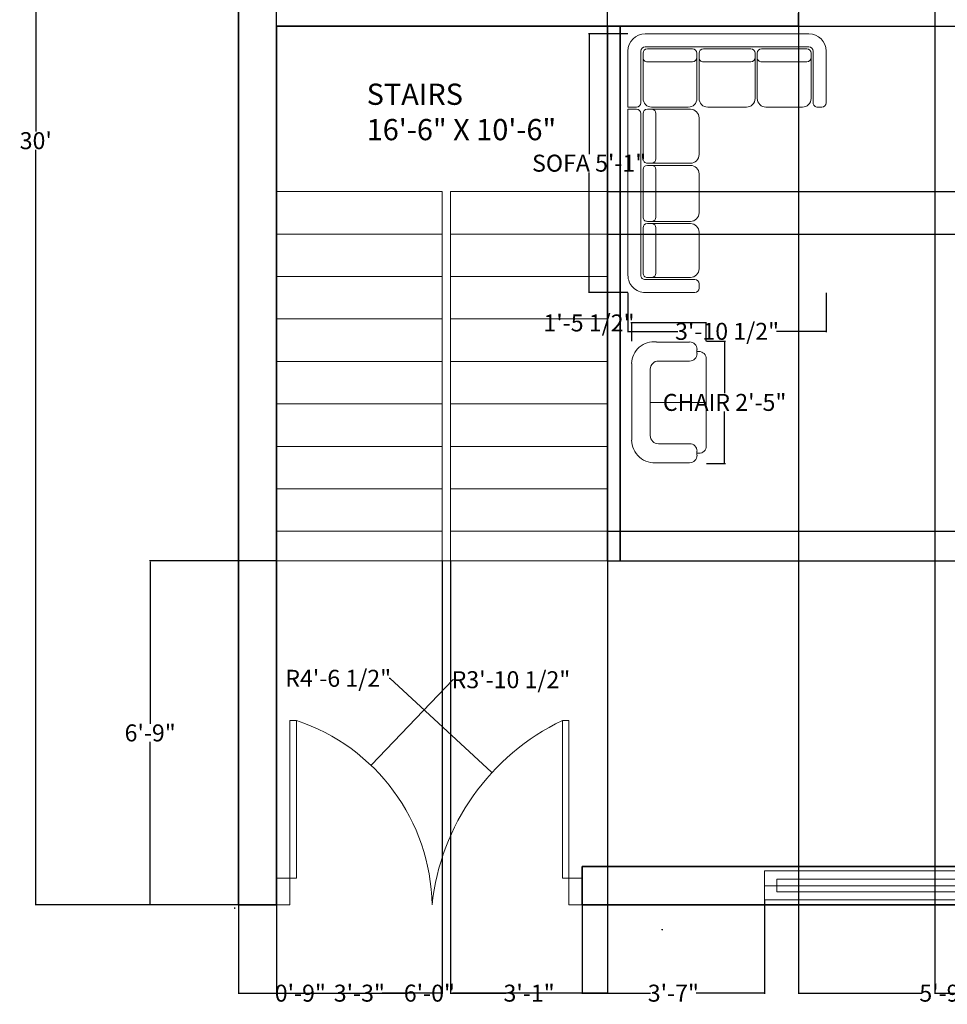
# Model space of a CAD drawing. Units: inches. Extents: x 311 to 754, y 60 to 497.
# Tile 1 of 11: x 311 to 530, y 64 to 296. Entities that reach past the tile are written whole.
import ezdxf

# ---------------------------------------------------------------- set-up
doc = ezdxf.new("R2010")
doc.units = ezdxf.units.IN
doc.header["$MEASUREMENT"] = 0
for name, color, linetype, lineweight in [('A-ANNO-DIMS', 2, 'Continuous', 18), ('A-AREA-IDEN', 1, 'Continuous', 18), ('A-FURN', 70, 'Continuous', 13), ('A-WALL', 7, 'Continuous', 35), ('doors', 210, 'Continuous', 18), ('stairs', 130, 'Continuous', 18), ('windows', 120, 'Continuous', 18)]:
    doc.layers.add(name, color=color, linetype=linetype, lineweight=lineweight)
doc.styles.get("Standard").update_dxf_attribs({"font": 'arial.ttf'})
doc.dimstyles.get("Standard").update_dxf_attribs({"dimtxt": 4, "dimasz": 0.18, "dimexe": 0.18, "dimexo": 0.0625, "dimgap": 0.09, "dimtad": 0, "dimtih": 1, "dimtoh": 1, "dimdec": 0, "dimrnd": 6, "dimzin": 0, "dimdsep": 46, "dimlunit": 3, "dimtxsty": 'Standard', "dimcen": 0.09, "dimadec": 0, "dimazin": 0, "dimtfac": 1, "dimtdec": 0, "dimtofl": 0, "dimtmove": 0, "dimatfit": 3, "dimfxl": 1, "dimtolj": 1, "dimtzin": 0, "dimarcsym": 0})

# ---------------------------------------------------------------- blocks, each defined once
blk = doc.blocks.new('A$C2AFA021D')
for p, q in [((0.8, 2.3), (0.2, 2.3)), ((0.85, 2.2), (0.85, 2.25)), ((0, 2.1), (0, 0.2)), ((0.15, 0.2), (0.15, 2.1)), ((0.175, 1.55), (0.175, 2.075)), ((0.2, 2.15), (0.8, 2.15)), ((0.225, 2.125), (0.275, 2.125)), ((0.75, 2.125), (0.275, 2.125)), ((0.325, 2.075), (0.325, 1.55)), ((0.85, 1.6), (0.85, 2.025)), ((0.275, 1.5), (0.225, 1.5)), ((0.275, 1.5), (0.75, 1.5)), ((0.175, 0.875), (0.175, 1.425)), ((0.225, 1.475), (0.275, 1.475)), ((0.75, 1.475), (0.275, 1.475)), ((0.325, 1.425), (0.325, 0.875)), ((0.85, 0.925), (0.85, 1.375)), ((0.275, 0.825), (0.225, 0.825)), ((0.225, 0.8), (0.275, 0.8)), ((0.275, 0.825), (0.75, 0.825)), ((0.75, 0.8), (0.275, 0.8)), ((0.975, 0.825), (1.4, 0.825)), ((1.625, 0.825), (2.075, 0.825)), ((2.3, 0.825), (2.725, 0.825)), ((2.9, 0.825), (2.95, 0.825)), ((0.175, 0.225), (0.175, 0.75)), ((0.325, 0.75), (0.325, 0.225)), ((0.85, 0.275), (0.85, 0.7)), ((0.875, 0.275), (0.875, 0.725)), ((1.5, 0.725), (1.5, 0.275)), ((1.525, 0.275), (1.525, 0.725)), ((2.175, 0.725), (2.175, 0.275)), ((2.2, 0.275), (2.2, 0.725)), ((2.825, 0.725), (2.825, 0.275)), ((2.85, 0.2), (2.85, 0.775)), ((3, 0.775), (3, 0.2)), ((0.875, 0.275), (0.875, 0.225)), ((1.45, 0.325), (0.925, 0.325)), ((1.5, 0.225), (1.5, 0.275)), ((1.525, 0.275), (1.525, 0.225)), ((2.125, 0.325), (1.575, 0.325)), ((2.175, 0.225), (2.175, 0.275)), ((2.2, 0.275), (2.2, 0.225)), ((2.775, 0.325), (2.25, 0.325)), ((2.825, 0.225), (2.825, 0.275)), ((0.8, 0.15), (0.2, 0.15)), ((0.275, 0.175), (0.225, 0.175)), ((0.275, 0.175), (0.75, 0.175)), ((0.925, 0.175), (1.45, 0.175)), ((0.925, 0.15), (2.8, 0.15)), ((1.575, 0.175), (2.125, 0.175)), ((2.25, 0.175), (2.775, 0.175)), ((0.85, 0), (0.85, 0.1)), ((0.875, 0.1), (0.875, 0)), ((0.2, 0), (0.85, 0)), ((2.8, 0), (0.875, 0))]:
    blk.add_line(p, q)
for centre, radius, start, end in [((0.2, 2.1), 0.2, 90, 180), ((0.8, 2.25), 0.05, 0, 90), ((0.8, 2.2), 0.05, 270, 0), ((0.2, 2.1), 0.05, 90, 180), ((0.225, 2.075), 0.05, 90, 180), ((0.275, 2.075), 0.05, 0, 90), ((0.75, 2.025), 0.1, 0, 90), ((0.75, 1.6), 0.1, 270, 0), ((0.225, 1.55), 0.05, 180, 270), ((0.275, 1.55), 0.05, 270, 0), ((0.225, 1.425), 0.05, 90, 180), ((0.275, 1.425), 0.05, 0, 90), ((0.75, 1.375), 0.1, 360, 90), ((0.75, 0.925), 0.1, 270, 0), ((0.225, 0.875), 0.05, 180, 270), ((0.225, 0.75), 0.05, 90, 180), ((0.275, 0.875), 0.05, 270, 0), ((0.275, 0.75), 0.05, 0, 90), ((0.75, 0.7), 0.1, 0, 90), ((0.975, 0.725), 0.1, 90, 180), ((1.4, 0.725), 0.1, 0, 90), ((1.625, 0.725), 0.1, 90, 180), ((2.075, 0.725), 0.1, 0, 90), ((2.3, 0.725), 0.1, 90, 180), ((2.725, 0.725), 0.1, 0, 90), ((2.9, 0.775), 0.05, 90, 180), ((2.95, 0.775), 0.05, 0, 90), ((0.75, 0.275), 0.1, 270, 0), ((0.925, 0.275), 0.05, 90, 180), ((1.45, 0.275), 0.05, 360, 90), ((1.575, 0.275), 0.05, 90, 180), ((2.125, 0.275), 0.05, 360, 90), ((2.25, 0.275), 0.05, 90, 180), ((2.775, 0.275), 0.05, 360, 90), ((0.2, 0.2), 0.2, 180, 270), ((0.2, 0.2), 0.05, 180, 270), ((0.225, 0.225), 0.05, 180, 270), ((0.275, 0.225), 0.05, 270, 0), ((0.8, 0.1), 0.05, 0, 90), ((0.925, 0.225), 0.05, 180, 270), ((0.925, 0.1), 0.05, 90, 180), ((1.45, 0.225), 0.05, 270, 0), ((1.575, 0.225), 0.05, 180, 270), ((2.125, 0.225), 0.05, 270, 0), ((2.25, 0.225), 0.05, 180, 270), ((2.775, 0.225), 0.05, 270, 0), ((2.8, 0.2), 0.2, 270, 0), ((2.8, 0.2), 0.05, 270, 0)]:
    blk.add_arc(centre, radius, start, end)
blk = doc.blocks.new('A$C6D011943')
for p, q in [((1.448, 1.089), (0.332, 1.089)), ((1.364, 0.818), (0.398, 0.818)), ((0.881, 0.818), (0.881, 0)), ((1.762, 0.247), (1.762, 0.727)), ((0, 0.709), (0, 0.247)), ((0.278, 0.697), (0.278, 0.244)), ((1.485, 0.244), (1.485, 0.697)), ((0.109, 0.136), (0.169, 0.136)), ((0.139, 0.109), (0.139, 0.136)), ((1.515, 0), (0.247, 0)), ((1.593, 0.136), (1.654, 0.136)), ((1.648, 0.136), (1.623, 0.136)), ((1.623, 0.109), (1.623, 0.136))]:
    blk.add_line(p, q)
for centre, radius, start, end in [((0.339, 0.748), 0.342, 91.2564, 186.501), ((1.441, 0.766), 0.324, 353.159, 88.6697), ((0.398, 0.697), 0.121, 90, 180), ((1.364, 0.697), 0.121, 0, 90), ((0.109, 0.244), 0.109, 180, 270), ((0.169, 0.244), 0.109, 270, 0), ((1.593, 0.244), 0.109, 180, 270), ((1.654, 0.244), 0.109, 270, 0), ((0.247, 0.109), 0.109, 180, 270), ((1.515, 0.109), 0.109, 270, 0)]:
    blk.add_arc(centre, radius, start, end)
blk = doc.blocks.new('*D104')
at = {"layer": 'A-ANNO-DIMS', "color": 0, "lineweight": -2, "transparency": 16777216}
for p, q in [((362.74, 447.24), (314.86, 447.24)), ((315.04, 447.06), (315.04, 269.37)), ((315.04, 87.42), (315.04, 265.1)), ((362.74, 87.24), (314.86, 87.24))]:
    blk.add_line(p, q, dxfattribs=at)
at = {"layer": 'A-ANNO-DIMS', "color": 0, "transparency": 16777216}
for points in [[(315.01, 447.06), (315.07, 447.06), (315.04, 447.24)], [(315.01, 87.42), (315.07, 87.42), (315.04, 87.24)]]:
    blk.add_solid(points, dxfattribs=at)
at = {"layer": 'Defpoints', "color": 0, "transparency": 16777216}
for p in [(362.8, 447.24), (315.04, 87.24), (362.8, 87.24)]:
    blk.add_point(p, dxfattribs=at)
at = {"layer": 'A-ANNO-DIMS', "color": 0, "transparency": 16777216, "insert": (315.04, 267.24), "char_height": 4, "attachment_point": 5}
blk.add_mtext("\\A1;30'", dxfattribs=at)
blk = doc.blocks.new('WIN-FRAME-59IN')
for points in [[(0, 0), (0, 6.8), (58.92, 6.8), (58.92, 0)], [(2.85, 4.84), (55.97, 4.84), (55.97, 1.89), (2.85, 1.89)]]:
    blk.add_lwpolyline(points, close=True)
blk = doc.blocks.new('*D114')
at = {"layer": 'A-ANNO-DIMS', "color": 0, "lineweight": -2, "transparency": 16777216}
for p, q in [((454.54, 292.4), (445.28, 292.4)), ((445.46, 292.22), (445.46, 264.1)), ((445.46, 231.65), (445.46, 259.78)), ((454.54, 231.47), (445.28, 231.47))]:
    blk.add_line(p, q, dxfattribs=at)
at = {"layer": 'A-ANNO-DIMS', "color": 0, "transparency": 16777216}
for points in [[(445.43, 292.22), (445.49, 292.22), (445.46, 292.4)], [(445.43, 231.65), (445.49, 231.65), (445.46, 231.47)]]:
    blk.add_solid(points, dxfattribs=at)
at = {"layer": 'Defpoints', "color": 0, "transparency": 16777216}
for p in [(454.6, 292.4), (445.46, 231.47), (454.6, 231.47)]:
    blk.add_point(p, dxfattribs=at)
at = {"layer": 'A-ANNO-DIMS', "color": 0, "transparency": 16777216, "insert": (445.46, 261.94), "char_height": 4, "attachment_point": 5}
blk.add_mtext('\\A1;SOFA 5\'-1"', dxfattribs=at)
blk = doc.blocks.new('*D115')
at = {"layer": 'A-ANNO-DIMS', "color": 0, "lineweight": -2, "transparency": 16777216}
for p, q in [((454.6, 231.41), (454.6, 222.15)), ((501.31, 231.41), (501.31, 222.15)), ((454.78, 222.33), (466.34, 222.33)), ((501.13, 222.33), (489.58, 222.33))]:
    blk.add_line(p, q, dxfattribs=at)
at = {"layer": 'A-ANNO-DIMS', "color": 0, "transparency": 16777216}
for points in [[(454.78, 222.36), (454.78, 222.3), (454.6, 222.33)], [(501.13, 222.36), (501.13, 222.3), (501.31, 222.33)]]:
    blk.add_solid(points, dxfattribs=at)
at = {"layer": 'Defpoints', "color": 0, "transparency": 16777216}
for p in [(454.6, 231.47), (501.31, 231.47), (501.31, 222.33)]:
    blk.add_point(p, dxfattribs=at)
at = {"layer": 'A-ANNO-DIMS', "color": 0, "transparency": 16777216, "insert": (477.96, 222.33), "char_height": 4, "attachment_point": 5}
blk.add_mtext('\\A1;3\'-10 1/2"', dxfattribs=at)
blk = doc.blocks.new('*D116')
at = {"layer": 'A-ANNO-DIMS', "color": 0, "lineweight": -2, "transparency": 16777216}
for p, q in [((473.13, 219.99), (477.56, 219.99)), ((477.38, 219.81), (477.38, 207.75)), ((477.38, 191.37), (477.38, 203.43)), ((473.13, 191.19), (477.56, 191.19))]:
    blk.add_line(p, q, dxfattribs=at)
at = {"layer": 'A-ANNO-DIMS', "color": 0, "transparency": 16777216}
for points in [[(477.35, 219.81), (477.41, 219.81), (477.38, 219.99)], [(477.35, 191.37), (477.41, 191.37), (477.38, 191.19)]]:
    blk.add_solid(points, dxfattribs=at)
at = {"layer": 'Defpoints', "color": 0, "transparency": 16777216}
for p in [(473.06, 219.99), (477.38, 219.99), (473.06, 191.19)]:
    blk.add_point(p, dxfattribs=at)
at = {"layer": 'A-ANNO-DIMS', "color": 0, "transparency": 16777216, "insert": (477.38, 205.59), "char_height": 4, "attachment_point": 5}
blk.add_mtext('\\A1;CHAIR 2\'-5"', dxfattribs=at)
blk = doc.blocks.new('*D117')
at = {"layer": 'A-ANNO-DIMS', "color": 0, "lineweight": -2, "transparency": 16777216}
for p, q in [((455.48, 224.31), (455.3, 224.31)), ((455.48, 220.05), (455.48, 224.49)), ((472.88, 224.31), (455.66, 224.31)), ((473.06, 220.05), (473.06, 224.49))]:
    blk.add_line(p, q, dxfattribs=at)
at = {"layer": 'A-ANNO-DIMS', "color": 0, "transparency": 16777216}
for points in [[(455.66, 224.34), (455.66, 224.28), (455.48, 224.31)], [(472.88, 224.34), (472.88, 224.28), (473.06, 224.31)]]:
    blk.add_solid(points, dxfattribs=at)
at = {"layer": 'Defpoints', "color": 0, "transparency": 16777216}
for p in [(455.48, 224.31), (455.48, 219.99), (473.06, 219.99)]:
    blk.add_point(p, dxfattribs=at)
at = {"layer": 'A-ANNO-DIMS', "color": 0, "transparency": 16777216, "insert": (445.42, 224.31), "char_height": 4, "attachment_point": 5}
blk.add_mtext('\\A1;1\'-5 1/2"', dxfattribs=at)
blk = doc.blocks.new('*D125')
at = {"layer": 'A-ANNO-DIMS', "color": 0, "lineweight": -2, "transparency": 16777216}
for p, q in [((371.8, 87.18), (371.8, 66.26)), ((443.8, 87.18), (443.8, 66.26)), ((371.98, 66.44), (402.39, 66.44)), ((443.62, 66.44), (413.22, 66.44))]:
    blk.add_line(p, q, dxfattribs=at)
at = {"layer": 'A-ANNO-DIMS', "color": 0, "transparency": 16777216}
for points in [[(371.98, 66.47), (371.98, 66.41), (371.8, 66.44)], [(443.62, 66.47), (443.62, 66.41), (443.8, 66.44)]]:
    blk.add_solid(points, dxfattribs=at)
at = {"layer": 'Defpoints', "color": 0, "transparency": 16777216}
for p in [(371.8, 87.24), (443.8, 87.24), (443.8, 66.44)]:
    blk.add_point(p, dxfattribs=at)
at = {"layer": 'A-ANNO-DIMS', "color": 0, "transparency": 16777216, "insert": (407.8, 66.44), "char_height": 4, "attachment_point": 5}
blk.add_mtext('\\A1;6\'-0"', dxfattribs=at)
blk = doc.blocks.new('*D126')
at = {"layer": 'A-ANNO-DIMS', "color": 0, "lineweight": -2, "transparency": 16777216}
for p, q in [((486.8, 88.36), (486.8, 66.26)), ((443.8, 87.18), (443.8, 66.26)), ((443.98, 66.44), (459.9, 66.44)), ((486.62, 66.44), (470.71, 66.44))]:
    blk.add_line(p, q, dxfattribs=at)
at = {"layer": 'A-ANNO-DIMS', "color": 0, "transparency": 16777216}
for points in [[(443.98, 66.47), (443.98, 66.41), (443.8, 66.44)], [(486.62, 66.47), (486.62, 66.41), (486.8, 66.44)]]:
    blk.add_solid(points, dxfattribs=at)
at = {"layer": 'Defpoints', "color": 0, "transparency": 16777216}
for p in [(486.8, 88.42), (443.8, 87.24), (486.8, 66.44)]:
    blk.add_point(p, dxfattribs=at)
at = {"layer": 'A-ANNO-DIMS', "color": 0, "transparency": 16777216, "insert": (465.3, 66.44), "char_height": 4, "attachment_point": 5}
blk.add_mtext('\\A1;3\'-7"', dxfattribs=at)
blk = doc.blocks.new('*D127')
at = {"layer": 'A-ANNO-DIMS', "color": 0, "lineweight": -2, "transparency": 16777216}
for p, q in [((371.74, 168.24), (341.82, 168.24)), ((342, 168.06), (342, 129.87)), ((342, 87.42), (342, 125.61)), ((362.74, 87.24), (341.82, 87.24))]:
    blk.add_line(p, q, dxfattribs=at)
at = {"layer": 'A-ANNO-DIMS', "color": 0, "transparency": 16777216}
for points in [[(341.97, 168.06), (342.03, 168.06), (342, 168.24)], [(341.97, 87.42), (342.03, 87.42), (342, 87.24)]]:
    blk.add_solid(points, dxfattribs=at)
at = {"layer": 'Defpoints', "color": 0, "transparency": 16777216}
for p in [(342, 168.24), (371.8, 168.24), (362.8, 87.24)]:
    blk.add_point(p, dxfattribs=at)
at = {"layer": 'A-ANNO-DIMS', "color": 0, "transparency": 16777216, "insert": (342, 127.74), "char_height": 4, "attachment_point": 5}
blk.add_mtext('\\A1;6\'-9"', dxfattribs=at)
blk = doc.blocks.new('*D128')
at = {"layer": 'A-ANNO-DIMS', "color": 0, "lineweight": -2, "transparency": 16777216}
for p, q in [((362.8, 87.18), (362.8, 66.26)), ((371.8, 87.18), (371.8, 66.26)), ((362.98, 66.44), (371.62, 66.44)), ((371.8, 66.44), (371.98, 66.44))]:
    blk.add_line(p, q, dxfattribs=at)
at = {"layer": 'A-ANNO-DIMS', "color": 0, "transparency": 16777216}
for points in [[(362.98, 66.47), (362.98, 66.41), (362.8, 66.44)], [(371.62, 66.47), (371.62, 66.41), (371.8, 66.44)]]:
    blk.add_solid(points, dxfattribs=at)
at = {"layer": 'Defpoints', "color": 0, "transparency": 16777216}
for p in [(362.8, 87.24), (371.8, 87.24), (371.8, 66.44)]:
    blk.add_point(p, dxfattribs=at)
at = {"layer": 'A-ANNO-DIMS', "color": 0, "transparency": 16777216, "insert": (377.39, 66.44), "char_height": 4, "attachment_point": 5}
blk.add_mtext('\\A1;0\'-9"', dxfattribs=at)
blk = doc.blocks.new('*D132')
at = {"layer": 'A-ANNO-DIMS', "color": 0, "lineweight": -2, "transparency": 16777216}
for p, q in [((526.91, 339.18), (526.91, 66.26)), ((560.82, 339.18), (560.82, 66.26)), ((527.09, 66.44), (536.87, 66.44)), ((560.64, 66.44), (550.86, 66.44))]:
    blk.add_line(p, q, dxfattribs=at)
at = {"layer": 'A-ANNO-DIMS', "color": 0, "transparency": 16777216}
for points in [[(527.09, 66.47), (527.09, 66.41), (526.91, 66.44)], [(560.64, 66.47), (560.64, 66.41), (560.82, 66.44)]]:
    blk.add_solid(points, dxfattribs=at)
at = {"layer": 'Defpoints', "color": 0, "transparency": 16777216}
for p in [(526.91, 339.24), (560.82, 339.24), (526.91, 66.44)]:
    blk.add_point(p, dxfattribs=at)
at = {"layer": 'A-ANNO-DIMS', "color": 0, "transparency": 16777216, "insert": (543.87, 66.44), "char_height": 4, "attachment_point": 5}
blk.add_mtext('\\A1;2\'-10"', dxfattribs=at)
blk = doc.blocks.new('*D134')
at = {"layer": 'A-ANNO-DIMS', "color": 0, "lineweight": -2, "transparency": 16777216}
for p, q in [((494.8, 342.18), (494.8, 66.26)), ((563.8, 342.18), (563.8, 66.26)), ((494.98, 66.44), (523.9, 66.44)), ((563.62, 66.44), (534.71, 66.44))]:
    blk.add_line(p, q, dxfattribs=at)
at = {"layer": 'A-ANNO-DIMS', "color": 0, "transparency": 16777216}
for points in [[(494.98, 66.47), (494.98, 66.41), (494.8, 66.44)], [(563.62, 66.47), (563.62, 66.41), (563.8, 66.44)]]:
    blk.add_solid(points, dxfattribs=at)
at = {"layer": 'Defpoints', "color": 0, "transparency": 16777216}
for p in [(494.8, 342.24), (563.8, 342.24), (563.8, 66.44)]:
    blk.add_point(p, dxfattribs=at)
at = {"layer": 'A-ANNO-DIMS', "color": 0, "transparency": 16777216, "insert": (529.3, 66.44), "char_height": 4, "attachment_point": 5}
blk.add_mtext('\\A1;5\'-9"', dxfattribs=at)
blk = doc.blocks.new('*D136')
at = {"layer": 'A-ANNO-DIMS', "color": 0, "lineweight": -2, "transparency": 16777216}
for p, q in [((371.8, 294.3), (371.8, 486.86)), ((371.98, 486.68), (405.39, 486.68)), ((449.62, 486.68), (416.22, 486.68)), ((449.8, 294.3), (449.8, 486.86))]:
    blk.add_line(p, q, dxfattribs=at)
at = {"layer": 'A-ANNO-DIMS', "color": 0, "transparency": 16777216}
for points in [[(371.98, 486.71), (371.98, 486.65), (371.8, 486.68)], [(449.62, 486.71), (449.62, 486.65), (449.8, 486.68)]]:
    blk.add_solid(points, dxfattribs=at)
at = {"layer": 'Defpoints', "color": 0, "transparency": 16777216}
for p in [(371.8, 486.68), (371.8, 294.24), (449.8, 294.24)]:
    blk.add_point(p, dxfattribs=at)
at = {"layer": 'A-ANNO-DIMS', "color": 0, "transparency": 16777216, "insert": (410.8, 486.68), "char_height": 4, "attachment_point": 5}
blk.add_mtext('\\A1;6\'-6"', dxfattribs=at)
blk = doc.blocks.new('*D137')
at = {"layer": 'A-ANNO-DIMS', "color": 0, "lineweight": -2, "transparency": 16777216}
for p, q in [((371.8, 168.18), (371.8, 66.26)), ((410.8, 168.18), (410.8, 66.26)), ((371.98, 66.44), (385.9, 66.44)), ((410.62, 66.44), (396.71, 66.44))]:
    blk.add_line(p, q, dxfattribs=at)
at = {"layer": 'A-ANNO-DIMS', "color": 0, "transparency": 16777216}
for points in [[(371.98, 66.47), (371.98, 66.41), (371.8, 66.44)], [(410.62, 66.47), (410.62, 66.41), (410.8, 66.44)]]:
    blk.add_solid(points, dxfattribs=at)
at = {"layer": 'Defpoints', "color": 0, "transparency": 16777216}
for p in [(371.8, 168.24), (410.8, 168.24), (371.8, 66.44)]:
    blk.add_point(p, dxfattribs=at)
at = {"layer": 'A-ANNO-DIMS', "color": 0, "transparency": 16777216, "insert": (391.3, 66.44), "char_height": 4, "attachment_point": 5}
blk.add_mtext('\\A1;3\'-3"', dxfattribs=at)
blk = doc.blocks.new('*D138')
at = {"layer": 'A-ANNO-DIMS', "color": 0, "lineweight": -2, "transparency": 16777216}
for p, q in [((412.8, 168.18), (412.8, 66.26)), ((449.8, 168.18), (449.8, 66.26)), ((412.98, 66.44), (425.9, 66.44)), ((449.62, 66.44), (436.71, 66.44))]:
    blk.add_line(p, q, dxfattribs=at)
at = {"layer": 'A-ANNO-DIMS', "color": 0, "transparency": 16777216}
for points in [[(412.98, 66.47), (412.98, 66.41), (412.8, 66.44)], [(449.62, 66.47), (449.62, 66.41), (449.8, 66.44)]]:
    blk.add_solid(points, dxfattribs=at)
at = {"layer": 'Defpoints', "color": 0, "transparency": 16777216}
for p in [(412.8, 168.24), (449.8, 168.24), (449.8, 66.44)]:
    blk.add_point(p, dxfattribs=at)
at = {"layer": 'A-ANNO-DIMS', "color": 0, "transparency": 16777216, "insert": (431.3, 66.44), "char_height": 4, "attachment_point": 5}
blk.add_mtext('\\A1;3\'-1"', dxfattribs=at)
blk = doc.blocks.new('*D139')
at = {"layer": 'A-ANNO-DIMS', "color": 0, "lineweight": -2, "transparency": 16777216}
for p, q in [((449.87, 255.24), (743.78, 255.24)), ((743.6, 255.06), (743.6, 252.37)), ((743.6, 245.42), (743.6, 248.11)), ((449.87, 245.24), (743.78, 245.24))]:
    blk.add_line(p, q, dxfattribs=at)
at = {"layer": 'A-ANNO-DIMS', "color": 0, "transparency": 16777216}
for points in [[(743.57, 255.06), (743.63, 255.06), (743.6, 255.24)], [(743.57, 245.42), (743.63, 245.42), (743.6, 245.24)]]:
    blk.add_solid(points, dxfattribs=at)
at = {"layer": 'Defpoints', "color": 0, "transparency": 16777216}
for p in [(449.8, 255.24), (743.6, 255.24), (449.8, 245.24)]:
    blk.add_point(p, dxfattribs=at)
at = {"layer": 'A-ANNO-DIMS', "color": 0, "transparency": 16777216, "insert": (743.6, 250.24), "char_height": 4, "attachment_point": 5}
blk.add_mtext('\\A1;0\'-10"', dxfattribs=at)
blk = doc.blocks.new('*D140')
at = {"layer": 'A-ANNO-DIMS', "color": 0, "lineweight": -2, "transparency": 16777216}
for p, q in [((449.87, 294.24), (743.78, 294.24)), ((743.6, 294.06), (743.6, 276.87)), ((743.6, 255.42), (743.6, 272.6)), ((449.87, 255.24), (743.78, 255.24))]:
    blk.add_line(p, q, dxfattribs=at)
at = {"layer": 'A-ANNO-DIMS', "color": 0, "transparency": 16777216}
for points in [[(743.57, 294.06), (743.63, 294.06), (743.6, 294.24)], [(743.57, 255.42), (743.63, 255.42), (743.6, 255.24)]]:
    blk.add_solid(points, dxfattribs=at)
at = {"layer": 'Defpoints', "color": 0, "transparency": 16777216}
for p in [(449.8, 294.24), (743.6, 294.24), (449.8, 255.24)]:
    blk.add_point(p, dxfattribs=at)
at = {"layer": 'A-ANNO-DIMS', "color": 0, "transparency": 16777216, "insert": (743.6, 274.74), "char_height": 4, "attachment_point": 5}
blk.add_mtext('\\A1;3\'-3"', dxfattribs=at)
blk = doc.blocks.new('*D141')
at = {"layer": 'A-ANNO-DIMS', "color": 0, "lineweight": -2, "transparency": 16777216}
for p, q in [((449.87, 175.24), (743.78, 175.24)), ((743.6, 175.06), (743.6, 173.87)), ((743.6, 168.42), (743.6, 169.61)), ((449.87, 168.24), (743.78, 168.24))]:
    blk.add_line(p, q, dxfattribs=at)
at = {"layer": 'A-ANNO-DIMS', "color": 0, "transparency": 16777216}
for points in [[(743.57, 175.06), (743.63, 175.06), (743.6, 175.24)], [(743.57, 168.42), (743.63, 168.42), (743.6, 168.24)]]:
    blk.add_solid(points, dxfattribs=at)
at = {"layer": 'Defpoints', "color": 0, "transparency": 16777216}
for p in [(449.8, 175.24), (743.6, 175.24), (449.8, 168.24)]:
    blk.add_point(p, dxfattribs=at)
at = {"layer": 'A-ANNO-DIMS', "color": 0, "transparency": 16777216, "insert": (743.6, 171.74), "char_height": 4, "attachment_point": 5}
blk.add_mtext('\\A1;0\'-7"', dxfattribs=at)
blk = doc.blocks.new('*D157')
at = {"layer": 'A-ANNO-DIMS', "color": 0, "lineweight": -2, "transparency": 16777216}
for p, q in [((413.32, 140.27), (394.18, 120.23)), ((413.5, 140.27), (413.32, 140.27)), ((361.86, 86.49), (362.04, 86.49)), ((361.95, 86.4), (361.95, 86.58))]:
    blk.add_line(p, q, dxfattribs=at)
at = {"layer": 'A-ANNO-DIMS', "color": 0, "transparency": 16777216}
blk.add_solid([(394.16, 120.26), (394.2, 120.21), (394.05, 120.1)], dxfattribs=at)
at = {"layer": 'Defpoints', "color": 0, "transparency": 16777216}
for p in [(394.05, 120.1), (361.95, 86.49)]:
    blk.add_point(p, dxfattribs=at)
at = {"layer": 'A-ANNO-DIMS', "color": 0, "transparency": 16777216, "insert": (427.03, 140.27), "char_height": 4, "attachment_point": 5}
blk.add_mtext('\\A1;R3\'-10 1/2"', dxfattribs=at)
blk = doc.blocks.new('*D158')
at = {"layer": 'A-ANNO-DIMS', "color": 0, "lineweight": -2, "transparency": 16777216}
for p, q in [((398.3, 140.6), (398.48, 140.6)), ((398.48, 140.6), (422.43, 118.52)), ((462.61, 81.41), (462.79, 81.41)), ((462.7, 81.32), (462.7, 81.5))]:
    blk.add_line(p, q, dxfattribs=at)
at = {"layer": 'A-ANNO-DIMS', "color": 0, "transparency": 16777216}
blk.add_solid([(422.45, 118.55), (422.41, 118.5), (422.56, 118.4)], dxfattribs=at)
at = {"layer": 'Defpoints', "color": 0, "transparency": 16777216}
for p in [(422.56, 118.4), (462.7, 81.41)]:
    blk.add_point(p, dxfattribs=at)
at = {"layer": 'A-ANNO-DIMS', "color": 0, "transparency": 16777216, "insert": (386.32, 140.6), "char_height": 4, "attachment_point": 5}
blk.add_mtext('\\A1;R4\'-6 1/2"', dxfattribs=at)

msp = doc.modelspace()

# ---------------------------------------------------------------- linework, layer by layer
at = {"layer": 'A-WALL'}
for p, q in [((362.8, 447.24), (362.8, 87.24)), ((494.8, 297.24), (494.8, 294.24)), ((494.8, 294.24), (371.8, 294.24)), ((371.8, 294.24), (371.8, 96.24)), ((449.8, 294.24), (449.8, 168.24)), ((452.8, 294.24), (452.8, 168.24)), ((371.8, 96.24), (371.8, 96.24)), ((371.8, 96.24), (371.8, 87.24)), ((443.8, 96.24), (590.8, 96.24)), ((443.8, 96.24), (443.8, 87.24)), ((362.8, 87.24), (371.8, 87.24)), ((443.8, 87.24), (722.8, 87.24))]:
    msp.add_line(p, q, dxfattribs=at)
at = {"layer": 'doors'}
for points in [[(374.94, 93.53), (376.46, 93.53), (376.46, 130.65), (374.94, 130.65)], [(439.15, 93.53), (440.67, 93.53), (440.67, 130.65), (439.15, 130.65)], [(371.8, 93.53), (371.8, 93.53), (371.8, 87.24), (371.8, 87.24)], [(371.8, 87.24), (374.94, 87.24), (374.94, 93.53), (371.8, 93.53)], [(440.67, 87.24), (443.8, 87.24), (443.8, 93.53), (440.67, 93.53)]]:
    msp.add_lwpolyline(points, close=True, dxfattribs=at)
for centre, radius, start, end in [((361.95, 86.49), 46.48, 0.923, 71.8091), ((462.7, 81.41), 54.59, 115.5638, 173.8668)]:
    msp.add_arc(centre, radius, start, end, dxfattribs=at)
at = {"layer": 'stairs'}
for p, q in [((371.8, 168.24), (371.8, 255.24)), ((371.8, 255.24), (410.8, 255.24)), ((410.8, 255.24), (410.8, 168.24)), ((412.8, 255.24), (412.8, 168.24)), ((412.8, 255.24), (449.8, 255.24)), ((449.8, 255.24), (449.8, 168.24)), ((371.8, 245.24), (410.8, 245.24)), ((412.8, 245.24), (449.8, 245.24)), ((371.8, 235.24), (410.8, 235.24)), ((412.8, 235.24), (449.8, 235.24)), ((371.8, 225.24), (410.8, 225.24)), ((412.8, 225.24), (449.8, 225.24)), ((371.8, 215.24), (410.8, 215.24)), ((412.8, 215.24), (449.8, 215.24)), ((371.8, 205.24), (410.8, 205.24)), ((412.8, 205.24), (449.8, 205.24)), ((371.8, 195.24), (410.8, 195.24)), ((412.8, 195.24), (449.8, 195.24)), ((371.8, 185.24), (410.8, 185.24)), ((412.8, 185.24), (449.8, 185.24)), ((371.8, 175.24), (410.8, 175.24)), ((412.8, 175.24), (449.8, 175.24)), ((452.8, 168.24), (371.8, 168.24)), ((449.8, 168.24), (371.8, 168.24))]:
    msp.add_line(p, q, dxfattribs=at)
at = {"layer": 'windows'}
msp.add_line((545.72, 91.7), (486.8, 91.7), dxfattribs=at)

# ---------------------------------------------------------------- block references
at = {"layer": 'A-FURN'}
for name, p, xscale, yscale, zscale, rotation in [('A$C2AFA021D', (454.6, 292.4), 20.30995506356601, 20.30995506356601, 20.30995506356601, 270), ('A$C6D011943', (473.06, 191.37), 16.14299049973071, 16.14299049973071, 16.14299049973071, 90)]:
    msp.add_blockref(name, p, dxfattribs=dict(at, xscale=xscale, yscale=yscale, zscale=zscale, rotation=rotation))
at = {"layer": 'windows'}
msp.add_blockref('WIN-FRAME-59IN', (486.8, 88.42), dxfattribs=at)

# ---------------------------------------------------------------- texts
at = {"layer": 'A-AREA-IDEN', "ltscale": 50, "insert": (393.02, 280.68), "char_height": 5, "attachment_point": 1}
msp.add_mtext_dynamic_manual_height_columns('STAIRS\\P16\'-6" X 10\'-6"\\P ', width=51.3734, gutter_width=1, heights=[0], dxfattribs=at)

# ---------------------------------------------------------------- dimensions: what is measured, and where the dimension line sits
at = {"layer": 'A-ANNO-DIMS'}
for base, p1, p2, picture, middle in [((371.8, 486.68), (449.8, 294.24), (371.8, 294.24), '*D136', (410.8, 486.68)), ((563.8, 66.44), (494.8, 342.24), (563.8, 342.24), '*D134', (529.3, 66.44)), ((526.91, 66.44), (560.82, 339.24), (526.91, 339.24), '*D132', (543.87, 66.44)), ((501.31, 222.33), (454.6, 231.47), (501.31, 231.47), '*D115', (477.96, 222.33)), ((371.8, 66.44), (410.8, 168.24), (371.8, 168.24), '*D137', (391.3, 66.44)), ((449.8, 66.44), (412.8, 168.24), (449.8, 168.24), '*D138', (431.3, 66.44)), ((486.8, 66.44), (443.8, 87.24), (486.8, 88.42), '*D126', (465.3, 66.44)), ((371.8, 66.44), (362.8, 87.24), (371.8, 87.24), '*D128', (377.39, 66.44)), ((443.8, 66.44), (371.8, 87.24), (443.8, 87.24), '*D125', (407.8, 66.44))]:
    dim = msp.add_linear_dim(base=base, p1=p1, p2=p2, dimstyle='Standard', override={"dimdec": 1, "dimlfac": 1, "dimrnd": 0, "dimzin": 1, "dimdsep": 46, "dimlunit": 4, "dimfrac": 2}, dxfattribs=at)
    dim.commit()
    dim.dimension.update_dxf_attribs({"geometry": picture, "text_midpoint": middle})
for base, p1, p2, angle, override, picture, middle in [((315.04, 87.24), (362.8, 447.24), (362.8, 87.24), 90, {"dimclrd": 0, "dimclre": 0, "dimclrt": 0}, '*D104', (315.04, 267.24)), ((743.6, 294.24), (449.8, 255.24), (449.8, 294.24), 90, {"dimdec": 1, "dimlfac": 1, "dimrnd": 0, "dimzin": 1, "dimdsep": 46, "dimlunit": 4, "dimfrac": 2}, '*D140', (743.6, 274.74)), ((743.6, 255.24), (449.8, 245.24), (449.8, 255.24), 90, {"dimdec": 1, "dimlfac": 1, "dimrnd": 0, "dimzin": 1, "dimdsep": 46, "dimlunit": 4, "dimfrac": 2}, '*D139', (743.6, 250.24)), ((455.48, 224.31), (473.06, 219.99), (455.48, 219.99), 180, {"dimdec": 1, "dimlfac": 1, "dimrnd": 0, "dimzin": 1, "dimdsep": 46, "dimlunit": 4, "dimfrac": 2}, '*D117', (445.42, 224.31)), ((743.6, 175.24), (449.8, 168.24), (449.8, 175.24), 90, {"dimdec": 1, "dimlfac": 1, "dimrnd": 0, "dimzin": 1, "dimdsep": 46, "dimlunit": 4, "dimfrac": 2}, '*D141', (743.6, 171.74)), ((342, 168.24), (362.8, 87.24), (371.8, 168.24), 90, {"dimdec": 1, "dimlfac": 1, "dimrnd": 0, "dimzin": 1, "dimdsep": 46, "dimlunit": 4, "dimfrac": 2}, '*D127', (342, 127.74))]:
    dim = msp.add_linear_dim(base=base, p1=p1, p2=p2, angle=angle, dimstyle='Standard', override=override, dxfattribs=at)
    dim.commit()
    dim.dimension.update_dxf_attribs({"geometry": picture, "text_midpoint": middle})
for base, p1, p2, angle, text, picture, middle in [((445.46, 231.47), (454.6, 292.4), (454.6, 231.47), 270, 'SOFA <>', '*D114', (445.46, 261.94)), ((477.38, 219.99), (473.06, 191.19), (473.06, 219.99), 90, 'CHAIR <>', '*D116', (477.38, 205.59))]:
    dim = msp.add_linear_dim(base=base, p1=p1, p2=p2, angle=angle, text=text, dimstyle='Standard', override={"dimdec": 1, "dimlfac": 1, "dimrnd": 0, "dimzin": 1, "dimdsep": 46, "dimlunit": 4, "dimfrac": 2}, dxfattribs=at)
    dim.commit()
    dim.dimension.update_dxf_attribs({"geometry": picture, "text_midpoint": middle})
for center, mpoint, picture, middle in [((361.95, 86.49), (394.05, 120.1), '*D157', (427.03, 140.27)), ((462.7, 81.41), (422.56, 118.4), '*D158', (386.32, 140.6))]:
    dim = msp.add_radius_dim(center=center, mpoint=mpoint, dimstyle='Standard', override={"dimdec": 1, "dimlfac": 1, "dimrnd": 0, "dimzin": 1, "dimdsep": 46, "dimlunit": 4, "dimfrac": 2}, dxfattribs=at)
    dim.commit()
    dim.dimension.update_dxf_attribs({"geometry": picture, "text_midpoint": middle, "dimtype": 164})

doc.saveas('drawing.dxf')
